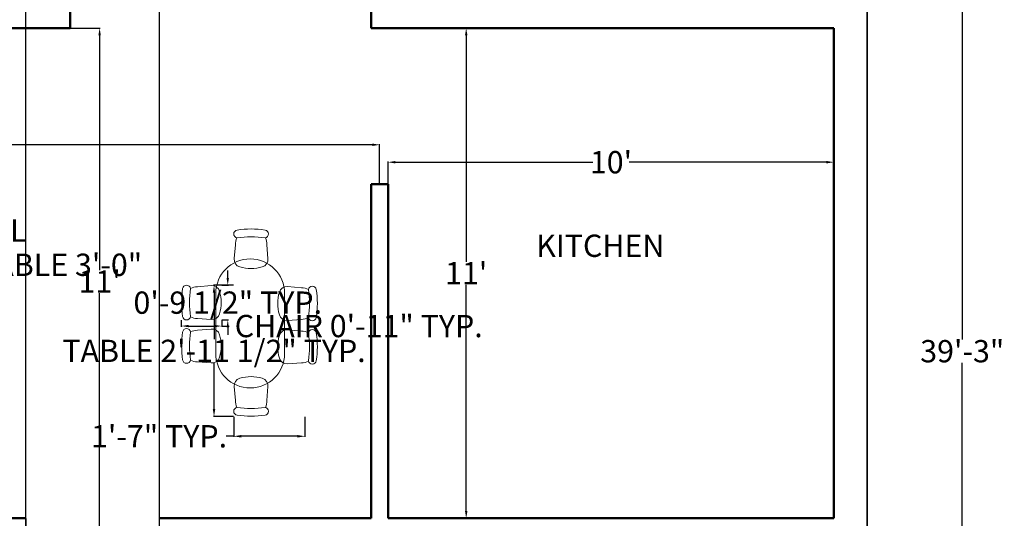
# Model space of a CAD drawing. Units: inches. Extents: x 134 to 568, y 15 to 554.
# Tile 6 of 7: x 303 to 568, y 235 to 369. Entities that reach past the tile are written whole.
import ezdxf

# ---------------------------------------------------------------- set-up
doc = ezdxf.new("R2010")
doc.units = ezdxf.units.IN
doc.header["$MEASUREMENT"] = 0
for name, color, linetype, lineweight in [('A-ANNO-DIMS', 2, 'Continuous', 18), ('A-AREA-IDEN', 7, 'Continuous', 25), ('A-FURN', 9, 'Continuous', 18), ('A-WALL', 7, 'Continuous', 50), ('C-PROP', 7, 'Continuous', 35)]:
    doc.layers.add(name, color=color, linetype=linetype, lineweight=lineweight)
doc.styles.add('ATT', font='TXT')
doc.styles.get("Standard").update_dxf_attribs({"font": 'arial.ttf'})
doc.dimstyles.get("Standard").update_dxf_attribs({"dimtxt": 6, "dimasz": 2, "dimexe": 0.18, "dimexo": 0.0625, "dimgap": 0.09, "dimtad": 0, "dimtih": 1, "dimtoh": 1, "dimdec": 0, "dimzin": 0, "dimdsep": 46, "dimlunit": 4, "dimtxsty": 'Standard', "dimcen": 0.09, "dimadec": 0, "dimazin": 0, "dimtfac": 1, "dimtdec": 0, "dimtofl": 0, "dimtmove": 0, "dimatfit": 3, "dimfxl": 1, "dimtolj": 1, "dimtzin": 0, "dimarcsym": 0})

# ---------------------------------------------------------------- blocks, each defined once
blk = doc.blocks.new('*D22')
at = {"layer": 'A-ANNO-DIMS', "color": 0, "lineweight": -2, "transparency": 16777216}
for p, q in [((179.83, 325.14), (179.83, 335.83)), ((181.83, 335.65), (279.72, 335.65)), ((397.83, 335.65), (299.95, 335.65)), ((399.83, 325.14), (399.83, 335.83))]:
    blk.add_line(p, q, dxfattribs=at)
at = {"layer": 'A-ANNO-DIMS', "color": 0, "transparency": 16777216}
for points in [[(181.83, 335.98), (181.83, 335.31), (179.83, 335.65)], [(397.83, 335.98), (397.83, 335.31), (399.83, 335.65)]]:
    blk.add_solid(points, dxfattribs=at)
at = {"layer": 'Defpoints', "color": 0, "transparency": 16777216}
for p in [(179.83, 335.65), (179.83, 325.08), (399.83, 325.08)]:
    blk.add_point(p, dxfattribs=at)
at = {"layer": 'A-ANNO-DIMS', "color": 0, "transparency": 16777216, "insert": (289.83, 335.65), "char_height": 6, "attachment_point": 5}
blk.add_mtext('\\A1;18\'-4"', dxfattribs=at)
blk = doc.blocks.new('*D23')
at = {"layer": 'A-ANNO-DIMS', "color": 0, "lineweight": -2, "transparency": 16777216}
for p, q in [((316.65, 367.08), (324.64, 367.08)), ((324.46, 365.08), (324.46, 301.93)), ((324.46, 232.58), (324.46, 295.73)), ((324.15, 230.58), (324.64, 230.58))]:
    blk.add_line(p, q, dxfattribs=at)
at = {"layer": 'A-ANNO-DIMS', "color": 0, "transparency": 16777216}
for points in [[(324.13, 365.08), (324.8, 365.08), (324.46, 367.08)], [(324.13, 232.58), (324.8, 232.58), (324.46, 230.58)]]:
    blk.add_solid(points, dxfattribs=at)
at = {"layer": 'Defpoints', "color": 0, "transparency": 16777216}
for p in [(316.58, 367.08), (324.08, 230.58), (324.46, 230.58)]:
    blk.add_point(p, dxfattribs=at)
at = {"layer": 'A-ANNO-DIMS', "color": 0, "transparency": 16777216, "insert": (324.46, 298.83), "char_height": 6, "attachment_point": 5}
blk.add_mtext("\\A1;11'", dxfattribs=at)
blk = doc.blocks.new('*D24')
at = {"layer": 'A-ANNO-DIMS', "color": 0, "lineweight": -2, "transparency": 16777216}
for p, q in [((402.15, 367.08), (423.3, 367.08)), ((423.12, 365.08), (423.12, 304.18)), ((423.12, 237.08), (423.12, 297.98)), ((402.15, 235.08), (423.3, 235.08))]:
    blk.add_line(p, q, dxfattribs=at)
at = {"layer": 'A-ANNO-DIMS', "color": 0, "transparency": 16777216}
for points in [[(422.79, 365.08), (423.46, 365.08), (423.12, 367.08)], [(422.79, 237.08), (423.46, 237.08), (423.12, 235.08)]]:
    blk.add_solid(points, dxfattribs=at)
at = {"layer": 'Defpoints', "color": 0, "transparency": 16777216}
for p in [(402.08, 367.08), (423.12, 367.08), (402.08, 235.08)]:
    blk.add_point(p, dxfattribs=at)
at = {"layer": 'A-ANNO-DIMS', "color": 0, "transparency": 16777216, "insert": (423.12, 301.08), "char_height": 6, "attachment_point": 5}
blk.add_mtext("\\A1;11'", dxfattribs=at)
blk = doc.blocks.new('*D25')
at = {"layer": 'A-ANNO-DIMS', "color": 0, "lineweight": -2, "transparency": 16777216}
for p, q in [((402.08, 325.14), (402.08, 331.14)), ((404.08, 330.96), (457.18, 330.96)), ((520.08, 330.96), (466.98, 330.96)), ((522.08, 325.14), (522.08, 331.14))]:
    blk.add_line(p, q, dxfattribs=at)
at = {"layer": 'A-ANNO-DIMS', "color": 0, "transparency": 16777216}
for points in [[(404.08, 331.29), (404.08, 330.63), (402.08, 330.96)], [(520.08, 331.29), (520.08, 330.63), (522.08, 330.96)]]:
    blk.add_solid(points, dxfattribs=at)
at = {"layer": 'Defpoints', "color": 0, "transparency": 16777216}
for p in [(522.08, 330.96), (402.08, 325.08), (522.08, 325.08)]:
    blk.add_point(p, dxfattribs=at)
at = {"layer": 'A-ANNO-DIMS', "color": 0, "transparency": 16777216, "insert": (462.08, 330.96), "char_height": 6, "attachment_point": 5}
blk.add_mtext("\\A1;10'", dxfattribs=at)
blk = doc.blocks.new('12PSTG01')
at = {"color": 0, "linetype": 'ByBlock'}
for p, q in [((-4.996459, 8.562867), (-11.998837, 7.942727)), ((-4.996459, -8.562867), (-11.998837, -8.055343))]:
    blk.add_line(p, q, dxfattribs=at)
for centre, radius, start, end in [((28, 0), 48, 171.544527, 188.455473), ((-17.5, 6.763875), 2, 8.455473, 171.544527), ((31.956522, 0), 48, 171.544527, 188.455473), ((-11.998837, -0.056308), 7.999035, 90, 116.212212), ((-4.647836, 4.578088), 4, 16.10866, 95), ((-20.5, 0), 20.5, 343.89134, 16.10866), ((-17.5, -6.763875), 2, 188.455473, 351.544527), ((-11.998837, -0.056308), 7.999035, 243.61801, 270), ((-4.647836, -4.578088), 4, 265, 343.89134)]:
    blk.add_arc(centre, radius, start, end, dxfattribs=at)
at = {"color": 0, "linetype": 'ByBlock', "style": 'ATT'}
for tag, p, flags in [('ITEM', (-19.5, -17.5), 3), ('ROOM_NUMBER', (-19.5, -25.5), 1)]:
    blk.add_attdef(tag, p, '', height=6, dxfattribs=dict(at, flags=flags))
blk = doc.blocks.new('-CHAI2')
at = {"xscale": 23, "yscale": 23, "zscale": 23}
blk.add_blockref('12PSTG01', (458, 200), dxfattribs=at)
blk = doc.blocks.new('*D40')
at = {"layer": 'A-ANNO-DIMS', "color": 0, "lineweight": -2, "transparency": 16777216}
for p, q in [((360.49, 297.85), (355.07, 297.85)), ((355.25, 295.85), (355.25, 283.36)), ((355.25, 264.48), (355.25, 276.97)), ((360.49, 262.48), (355.07, 262.48))]:
    blk.add_line(p, q, dxfattribs=at)
at = {"layer": 'A-ANNO-DIMS', "color": 0, "transparency": 16777216}
for points in [[(354.92, 295.85), (355.58, 295.85), (355.25, 297.85)], [(354.92, 264.48), (355.58, 264.48), (355.25, 262.48)]]:
    blk.add_solid(points, dxfattribs=at)
at = {"layer": 'Defpoints', "color": 0, "transparency": 16777216}
for p in [(355.25, 297.85), (360.56, 297.85), (360.56, 262.48)]:
    blk.add_point(p, dxfattribs=at)
at = {"layer": 'A-ANNO-DIMS', "color": 0, "transparency": 16777216, "insert": (355.25, 280.16), "char_height": 6, "attachment_point": 5}
blk.add_mtext('\\A1;TABLE 2\'-11 1/2" TYP.', dxfattribs=at)
blk = doc.blocks.new('*D41')
at = {"layer": 'A-ANNO-DIMS', "color": 0, "lineweight": -2, "transparency": 16777216}
for p, q in [((360.56, 262.42), (360.56, 256.99)), ((379.72, 262.42), (379.72, 256.99)), ((360.56, 257.17), (358.56, 257.17)), ((377.72, 257.17), (362.56, 257.17))]:
    blk.add_line(p, q, dxfattribs=at)
at = {"layer": 'A-ANNO-DIMS', "color": 0, "transparency": 16777216}
for points in [[(362.56, 257.51), (362.56, 256.84), (360.56, 257.17)], [(377.72, 257.51), (377.72, 256.84), (379.72, 257.17)]]:
    blk.add_solid(points, dxfattribs=at)
at = {"layer": 'Defpoints', "color": 0, "transparency": 16777216}
for p in [(360.56, 262.48), (379.72, 262.48), (360.56, 257.17)]:
    blk.add_point(p, dxfattribs=at)
at = {"layer": 'A-ANNO-DIMS', "color": 0, "transparency": 16777216, "insert": (340.46, 257.17), "char_height": 6, "attachment_point": 5}
blk.add_mtext('\\A1;1\'-7" TYP.', dxfattribs=at)
blk = doc.blocks.new('*D42')
at = {"layer": 'A-ANNO-DIMS', "color": 0, "lineweight": -2, "transparency": 16777216}
for p, q in [((346.43, 288.42), (346.43, 286.67)), ((348.43, 286.85), (355.32, 286.85)), ((357.32, 288.42), (357.32, 286.67)), ((357.32, 286.85), (359.32, 286.85))]:
    blk.add_line(p, q, dxfattribs=at)
at = {"layer": 'A-ANNO-DIMS', "color": 0, "transparency": 16777216}
for points in [[(348.43, 287.18), (348.43, 286.52), (346.43, 286.85)], [(355.32, 287.18), (355.32, 286.52), (357.32, 286.85)]]:
    blk.add_solid(points, dxfattribs=at)
at = {"layer": 'Defpoints', "color": 0, "transparency": 16777216}
for p in [(346.43, 288.48), (357.32, 288.48), (357.32, 286.85)]:
    blk.add_point(p, dxfattribs=at)
at = {"layer": 'A-ANNO-DIMS', "color": 0, "transparency": 16777216, "insert": (394.19, 286.85), "char_height": 6, "attachment_point": 5}
blk.add_mtext('\\A1;CHAIR 0\'-11" TYP.', dxfattribs=at)
blk = doc.blocks.new('*D43')
at = {"layer": 'A-ANNO-DIMS', "color": 0, "lineweight": -2, "transparency": 16777216}
for p, q in [((358.95, 299.82), (358.95, 301.82)), ((357.38, 297.82), (359.13, 297.82)), ((357.38, 288.48), (359.13, 288.48)), ((358.95, 286.48), (358.95, 284.48))]:
    blk.add_line(p, q, dxfattribs=at)
at = {"layer": 'A-ANNO-DIMS', "color": 0, "transparency": 16777216}
for points in [[(358.62, 299.82), (359.28, 299.82), (358.95, 297.82)], [(358.62, 286.48), (359.28, 286.48), (358.95, 288.48)]]:
    blk.add_solid(points, dxfattribs=at)
at = {"layer": 'Defpoints', "color": 0, "transparency": 16777216}
for p in [(357.32, 297.82), (358.95, 297.82), (357.32, 288.48)]:
    blk.add_point(p, dxfattribs=at)
at = {"layer": 'A-ANNO-DIMS', "color": 0, "transparency": 16777216, "insert": (358.95, 293.15), "char_height": 6, "attachment_point": 5}
blk.add_mtext('\\A1;0\'-9 1/2" TYP.', dxfattribs=at)
blk = doc.blocks.new('*D46')
at = {"layer": 'A-ANNO-DIMS', "color": 0, "lineweight": -2, "transparency": 16777216}
for p, q in [((232.99, 298.03), (232.99, 303.52)), ((234.99, 303.34), (266.85, 303.34)), ((268.85, 298.03), (268.85, 303.52)), ((268.85, 303.34), (270.85, 303.34))]:
    blk.add_line(p, q, dxfattribs=at)
at = {"layer": 'A-ANNO-DIMS', "color": 0, "transparency": 16777216}
for points in [[(234.99, 303.68), (234.99, 303.01), (232.99, 303.34)], [(266.85, 303.68), (266.85, 303.01), (268.85, 303.34)]]:
    blk.add_solid(points, dxfattribs=at)
at = {"layer": 'Defpoints', "color": 0, "transparency": 16777216}
for p in [(268.85, 303.34), (232.99, 297.97), (268.85, 297.97)]:
    blk.add_point(p, dxfattribs=at)
at = {"layer": 'A-ANNO-DIMS', "color": 0, "transparency": 16777216, "insert": (303.93, 303.34), "char_height": 6, "attachment_point": 5}
blk.add_mtext('\\A1;LOW TABLE 3\'-0"', dxfattribs=at)
blk = doc.blocks.new('*D60')
at = {"layer": 'A-ANNO-DIMS', "color": 0, "lineweight": -2, "transparency": 16777216}
for p, q in [((522.15, 515.58), (556.81, 515.58)), ((556.63, 513.58), (556.63, 283.24)), ((556.63, 46.58), (556.63, 276.93)), ((522.15, 44.58), (556.81, 44.58))]:
    blk.add_line(p, q, dxfattribs=at)
at = {"layer": 'A-ANNO-DIMS', "color": 0, "transparency": 16777216}
for points in [[(556.3, 513.58), (556.97, 513.58), (556.63, 515.58)], [(556.3, 46.58), (556.97, 46.58), (556.63, 44.58)]]:
    blk.add_solid(points, dxfattribs=at)
at = {"layer": 'Defpoints', "color": 0, "transparency": 16777216}
for p in [(522.08, 515.58), (556.63, 515.58), (522.08, 44.58)]:
    blk.add_point(p, dxfattribs=at)
at = {"layer": 'A-ANNO-DIMS', "color": 0, "transparency": 16777216, "insert": (556.63, 280.08), "char_height": 6, "attachment_point": 5}
blk.add_mtext('\\A1;39\'-3"', dxfattribs=at)
blk = doc.blocks.new('*D63')
at = {"layer": 'A-ANNO-DIMS', "color": 0, "lineweight": -2, "transparency": 16777216}
for p, q in [((304.58, 114.64), (304.58, 550.31)), ((306.58, 550.13), (314.52, 550.13)), ((338.58, 550.13), (330.65, 550.13)), ((340.58, 114.64), (340.58, 550.31))]:
    blk.add_line(p, q, dxfattribs=at)
at = {"layer": 'A-ANNO-DIMS', "color": 0, "transparency": 16777216}
for points in [[(306.58, 550.47), (306.58, 549.8), (304.58, 550.13)], [(338.58, 550.47), (338.58, 549.8), (340.58, 550.13)]]:
    blk.add_solid(points, dxfattribs=at)
at = {"layer": 'Defpoints', "color": 0, "transparency": 16777216}
for p in [(340.58, 550.13), (304.58, 114.58), (340.58, 114.58)]:
    blk.add_point(p, dxfattribs=at)
at = {"layer": 'A-ANNO-DIMS', "color": 0, "transparency": 16777216, "insert": (322.58, 550.13), "char_height": 6, "attachment_point": 5}
blk.add_mtext('\\A1;3\'-0"', dxfattribs=at)
blk = doc.blocks.new('*D64')
at = {"layer": 'A-ANNO-DIMS', "color": 0, "lineweight": -2, "transparency": 16777216}
for p, q in [((304.58, 235.02), (304.58, 18.85)), ((340.58, 230.52), (340.58, 18.85)), ((306.58, 19.03), (314.52, 19.03)), ((338.58, 19.03), (330.65, 19.03))]:
    blk.add_line(p, q, dxfattribs=at)
at = {"layer": 'A-ANNO-DIMS', "color": 0, "transparency": 16777216}
for points in [[(306.58, 19.37), (306.58, 18.7), (304.58, 19.03)], [(338.58, 19.37), (338.58, 18.7), (340.58, 19.03)]]:
    blk.add_solid(points, dxfattribs=at)
at = {"layer": 'Defpoints', "color": 0, "transparency": 16777216}
for p in [(304.58, 235.08), (340.58, 230.58), (340.58, 19.03)]:
    blk.add_point(p, dxfattribs=at)
at = {"layer": 'A-ANNO-DIMS', "color": 0, "transparency": 16777216, "insert": (322.58, 19.03), "char_height": 6, "attachment_point": 5}
blk.add_mtext('\\A1;3\'-0"', dxfattribs=at)

msp = doc.modelspace()

# ---------------------------------------------------------------- linework, layer by layer
at = {"layer": 'A-FURN'}
for p, q in [((355.72, 295.65), (355.72, 279.44)), ((374.25, 295.65), (374.25, 279.44))]:
    msp.add_line(p, q, dxfattribs=at)
for centre, start, end in [((364.99, 295.65), 0, 180), ((364.99, 279.44), 180, 0)]:
    msp.add_arc(centre, 9.26, start, end, dxfattribs=at)
at = {"layer": 'A-WALL'}
for p, q in [((316.58, 371.58), (316.58, 367.08)), ((397.58, 367.08), (397.58, 371.58)), ((180.08, 367.08), (316.58, 367.08)), ((397.58, 367.08), (522.08, 367.08)), ((522.08, 235.08), (522.08, 367.08)), ((397.58, 235.08), (397.58, 325.08)), ((397.58, 325.08), (402.08, 325.08)), ((402.08, 235.08), (402.08, 325.08)), ((300.08, 235.08), (304.58, 235.08)), ((340.58, 235.08), (397.58, 235.08)), ((402.08, 235.08), (522.08, 235.08))]:
    msp.add_line(p, q, dxfattribs=at)
at = {"layer": 'C-PROP'}
msp.add_line((531.08, 44.58), (531.08, 524.58), dxfattribs=at)

# ---------------------------------------------------------------- block references
at = {"layer": 'A-FURN', "extrusion": (0, 0, -1), "xscale": 0.5325640655624805, "yscale": 0.5325640655624805, "zscale": -0.5325640655618535, "rotation": 270}
msp.add_blockref('12PSTG01', (-365.22, 302.33), dxfattribs=at)
at = {"layer": 'A-FURN', "xscale": 0.0231549593732279, "yscale": 0.0231549593732279, "zscale": 0.0231549593732279}
for p in [(346.58, 288.53), (346.58, 276.85)]:
    msp.add_blockref('-CHAI2', p, dxfattribs=at)
at = {"layer": 'A-FURN', "extrusion": (0, 0, -1), "xscale": 0.5325640655589706, "yscale": 0.5325640655589706, "zscale": -0.5325640655618535}
for p in [(-372.41, 292.93), (-372.41, 281.25)]:
    msp.add_blockref('12PSTG01', p, dxfattribs=at)
at = {"layer": 'A-FURN', "xscale": 0.5325640655624805, "yscale": 0.5325640655624805, "zscale": 0.5325640655624805, "rotation": 90}
msp.add_blockref('12PSTG01', (365.22, 273.22), dxfattribs=at)

# ---------------------------------------------------------------- texts
at = {"layer": 'A-AREA-IDEN', "char_height": 6, "attachment_point": 1}
for s, width, insert in [('\\pxqc;HALL', 44.0209, (272.87, 315.59)), ('KITCHEN', 65.4319, (441.96, 311.46))]:
    msp.add_mtext_dynamic_manual_height_columns(s, width=width, gutter_width=30, heights=[0], dxfattribs=dict(at, insert=insert))

# ---------------------------------------------------------------- dimensions: what is measured, and where the dimension line sits
at = {"layer": 'A-ANNO-DIMS'}
for base, p1, p2, override, picture, middle in [((340.58, 550.13), (304.58, 114.58), (340.58, 114.58), {"dimdec": 1, "dimlfac": 1, "dimrnd": 0, "dimzin": 1, "dimdsep": 46, "dimlunit": 4, "dimfrac": 2}, '*D63', (322.58, 550.13)), ((179.83, 335.65), (399.83, 325.08), (179.83, 325.08), {"dimclrd": 0, "dimclre": 0, "dimclrt": 0}, '*D22', (289.83, 335.65)), ((522.08, 330.96), (402.08, 325.08), (522.08, 325.08), {"dimclrd": 0, "dimclre": 0, "dimclrt": 0}, '*D25', (462.08, 330.96)), ((340.58, 19.03), (304.58, 235.08), (340.58, 230.58), {"dimdec": 1, "dimlfac": 1, "dimrnd": 0, "dimzin": 1, "dimdsep": 46, "dimlunit": 4, "dimfrac": 2}, '*D64', (322.58, 19.03))]:
    dim = msp.add_linear_dim(base=base, p1=p1, p2=p2, dimstyle='Standard', override=override, dxfattribs=at)
    dim.commit()
    dim.dimension.update_dxf_attribs({"geometry": picture, "text_midpoint": middle})
for base, p1, p2, override, picture, middle in [((556.63, 515.58), (522.08, 44.58), (522.08, 515.58), {"dimdec": 1, "dimlfac": 1, "dimrnd": 0, "dimzin": 1, "dimdsep": 46, "dimlunit": 4, "dimfrac": 2}, '*D60', (556.63, 280.08)), ((423.12, 367.08), (402.08, 235.08), (402.08, 367.08), {"dimclrd": 0, "dimclre": 0, "dimclrt": 0}, '*D24', (423.12, 301.08))]:
    dim = msp.add_linear_dim(base=base, p1=p1, p2=p2, angle=90, dimstyle='Standard', override=override, dxfattribs=at)
    dim.commit()
    dim.dimension.update_dxf_attribs({"geometry": picture, "text_midpoint": middle})
for base, p1, p2, angle, text, override, picture, middle in [((324.46, 230.58), (316.58, 367.08), (324.08, 230.58), 90, "11'", {"dimclrd": 0, "dimclre": 0, "dimclrt": 0}, '*D23', (324.46, 298.83)), ((358.95, 297.82), (357.32, 288.48), (357.32, 297.82), 90, '<> TYP.', {"dimdec": 1, "dimlfac": 1, "dimrnd": 0, "dimzin": 1, "dimdsep": 46, "dimlunit": 4, "dimfrac": 2}, '*D43', (358.95, 293.15)), ((355.25, 297.85), (360.56, 262.48), (360.56, 297.85), 90, 'TABLE <> TYP.', {"dimdec": 1, "dimlfac": 1, "dimrnd": 0, "dimzin": 1, "dimdsep": 46, "dimlunit": 4, "dimfrac": 2}, '*D40', (355.25, 280.16)), ((360.56, 257.17), (379.72, 262.48), (360.56, 262.48), 180, '<> TYP.', {"dimdec": 1, "dimlfac": 1, "dimrnd": 0, "dimzin": 1, "dimdsep": 46, "dimlunit": 4, "dimfrac": 2}, '*D41', (340.46, 257.17))]:
    dim = msp.add_linear_dim(base=base, p1=p1, p2=p2, angle=angle, text=text, dimstyle='Standard', override=override, dxfattribs=at)
    dim.commit()
    dim.dimension.update_dxf_attribs({"geometry": picture, "text_midpoint": middle})
for base, p1, p2, text, picture, middle in [((268.85, 303.34), (232.99, 297.97), (268.85, 297.97), 'LOW TABLE <>', '*D46', (303.93, 303.34)), ((357.32, 286.85), (346.43, 288.48), (357.32, 288.48), 'CHAIR <> TYP.', '*D42', (394.19, 286.85))]:
    dim = msp.add_linear_dim(base=base, p1=p1, p2=p2, text=text, dimstyle='Standard', override={"dimdec": 1, "dimlfac": 1, "dimrnd": 0, "dimzin": 1, "dimdsep": 46, "dimlunit": 4, "dimfrac": 2}, dxfattribs=at)
    dim.commit()
    dim.dimension.update_dxf_attribs({"geometry": picture, "text_midpoint": middle})

doc.saveas('drawing.dxf')
